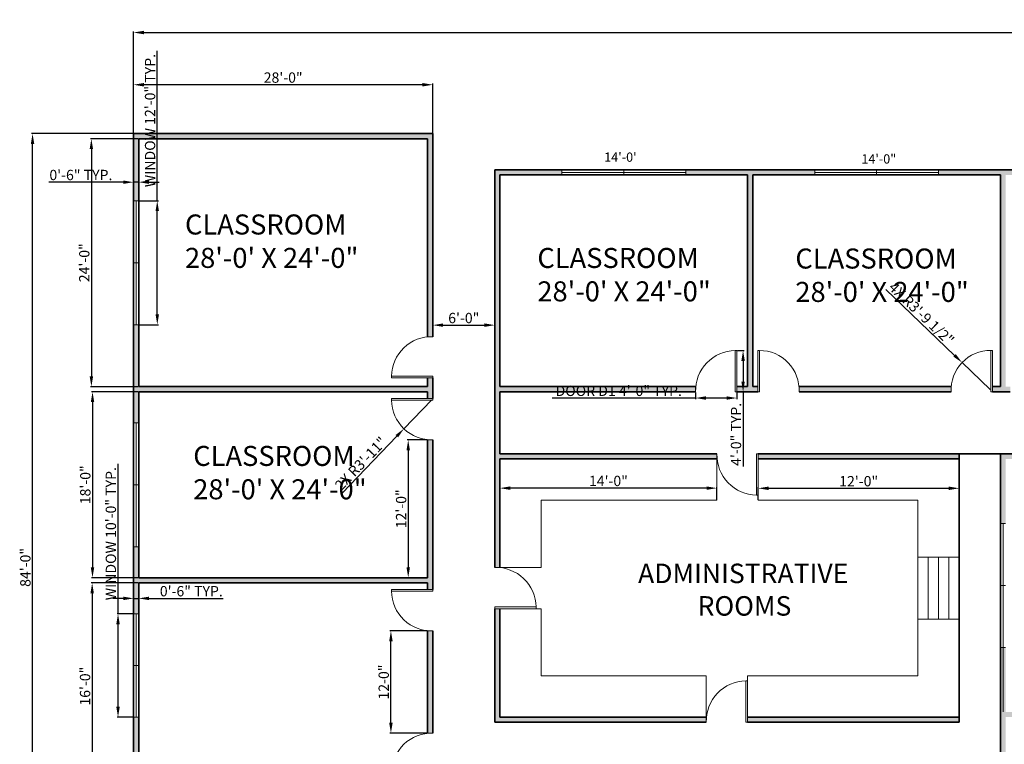
# Model space of a CAD drawing. Units: inches. Extents: x 2623 to 5095, y 1050 to 2384.
# Tile 2 of 4: x 2623 to 3768, y 1542 to 2384. Entities that reach past the tile are written whole.
import ezdxf

# ---------------------------------------------------------------- set-up
doc = ezdxf.new("R2010")
doc.units = ezdxf.units.IN
for name, color, linetype, lineweight in [('A-ANNO-DIMS', 2, 'Continuous', 13), ('A-ANNO-TEXT', 7, 'Continuous', 18), ('A-AREA-IDEN', 7, 'Continuous', 18), ('A-DOOR', 3, 'Continuous', 18), ('A-FLOR', 7, 'Continuous', 18), ('A-FLOR-STRS', 7, 'Continuous', 18), ('A-GLAZ', 4, 'Continuous', 18), ('A-WALL', 7, 'Continuous', 35)]:
    doc.layers.add(name, color=color, linetype=linetype, lineweight=lineweight)
doc.layers.add('A-WALL-PATT', color=251, linetype='Continuous', lineweight=9, true_color=0x636466)
doc.styles.get("Standard").update_dxf_attribs({"font": 'arial.ttf'})
doc.dimstyles.new('ISO-25', dxfattribs={"dimtxt": 12, "dimasz": 12, "dimexe": 1.25, "dimexo": 0.625, "dimtad": 1, "dimlunit": 3, "dimtxsty": 'Standard', "dimcen": 2.5, "dimadec": 0, "dimazin": 0, "dimtfac": 1, "dimtmove": 0, "dimatfit": 3, "dimfxl": 1, "dimarcsym": 0})

# ---------------------------------------------------------------- blocks, each defined once
blk = doc.blocks.new('*D8')
at = {"layer": 'A-ANNO-DIMS', "color": 0, "lineweight": -2, "transparency": 16777216}
for p, q in [((2755.7, 2252.2), (2755.7, 2309.7)), ((3091.7, 2308.4), (2767.7, 2308.4)), ((3103.7, 2252.2), (3103.7, 2309.7))]:
    blk.add_line(p, q, dxfattribs=at)
at = {"layer": 'A-ANNO-DIMS', "color": 0, "transparency": 16777216}
for points in [[(2767.7, 2310.4), (2767.7, 2306.4), (2755.7, 2308.4)], [(3091.7, 2310.4), (3091.7, 2306.4), (3103.7, 2308.4)]]:
    blk.add_solid(points, dxfattribs=at)
at = {"layer": 'Defpoints', "color": 0, "transparency": 16777216}
for p in [(2755.7, 2308.4), (2755.7, 2251.6), (3103.7, 2251.6)]:
    blk.add_point(p, dxfattribs=at)
at = {"layer": 'A-ANNO-DIMS', "color": 0, "transparency": 16777216, "insert": (2929.7, 2315.2), "char_height": 12, "attachment_point": 5}
blk.add_mtext('28\'-0"', dxfattribs=at)
blk = doc.blocks.new('*D9')
at = {"layer": 'A-ANNO-DIMS', "color": 0, "lineweight": -2, "transparency": 16777216}
for p, q in [((2761.1, 2245.6), (2705.5, 2245.6)), ((2706.7, 2233.6), (2706.7, 1969.6)), ((2761.1, 1957.6), (2705.5, 1957.6))]:
    blk.add_line(p, q, dxfattribs=at)
at = {"layer": 'A-ANNO-DIMS', "color": 0, "transparency": 16777216}
for points in [[(2704.7, 2233.6), (2708.7, 2233.6), (2706.7, 2245.6)], [(2704.7, 1969.6), (2708.7, 1969.6), (2706.7, 1957.6)]]:
    blk.add_solid(points, dxfattribs=at)
at = {"layer": 'Defpoints', "color": 0, "transparency": 16777216}
for p in [(2761.7, 2245.6), (2706.7, 1957.6), (2761.7, 1957.6)]:
    blk.add_point(p, dxfattribs=at)
at = {"layer": 'A-ANNO-DIMS', "color": 0, "transparency": 16777216, "insert": (2700, 2101.6), "char_height": 12, "attachment_point": 5, "rotation": 90}
blk.add_mtext('24\'-0"', dxfattribs=at)
blk = doc.blocks.new('*D10')
at = {"layer": 'A-ANNO-DIMS', "color": 0, "lineweight": -2, "transparency": 16777216}
for p, q in [((2761.1, 1951.6), (2706.7, 1951.6)), ((2708, 1939.6), (2708, 1747.6)), ((2761.1, 1735.6), (2706.7, 1735.6))]:
    blk.add_line(p, q, dxfattribs=at)
at = {"layer": 'A-ANNO-DIMS', "color": 0, "transparency": 16777216}
for points in [[(2706, 1939.6), (2710, 1939.6), (2708, 1951.6)], [(2706, 1747.6), (2710, 1747.6), (2708, 1735.6)]]:
    blk.add_solid(points, dxfattribs=at)
at = {"layer": 'Defpoints', "color": 0, "transparency": 16777216}
for p in [(2761.7, 1951.6), (2708, 1735.6), (2761.7, 1735.6)]:
    blk.add_point(p, dxfattribs=at)
at = {"layer": 'A-ANNO-DIMS', "color": 0, "transparency": 16777216, "insert": (2701.2, 1843.6), "char_height": 12, "attachment_point": 5, "rotation": 90}
blk.add_mtext('18\'-0"', dxfattribs=at)
blk = doc.blocks.new('*D11')
at = {"layer": 'A-ANNO-DIMS', "color": 0, "lineweight": -2, "transparency": 16777216}
for p, q in [((2761.1, 1729.6), (2706.4, 1729.6)), ((2707.6, 1717.6), (2707.6, 1501.6)), ((2761.1, 1489.6), (2706.4, 1489.6))]:
    blk.add_line(p, q, dxfattribs=at)
at = {"layer": 'A-ANNO-DIMS', "color": 0, "transparency": 16777216}
for points in [[(2705.6, 1717.6), (2709.6, 1717.6), (2707.6, 1729.6)], [(2705.6, 1501.6), (2709.6, 1501.6), (2707.6, 1489.6)]]:
    blk.add_solid(points, dxfattribs=at)
at = {"layer": 'Defpoints', "color": 0, "transparency": 16777216}
for p in [(2761.7, 1729.6), (2707.6, 1489.6), (2761.7, 1489.6)]:
    blk.add_point(p, dxfattribs=at)
at = {"layer": 'A-ANNO-DIMS', "color": 0, "transparency": 16777216, "insert": (2700.9, 1609.6), "char_height": 12, "attachment_point": 5, "rotation": 90}
blk.add_mtext('16\'-0"', dxfattribs=at)
blk = doc.blocks.new('*D22')
at = {"layer": 'A-ANNO-DIMS', "color": 0, "lineweight": -2, "transparency": 16777216}
for p, q in [((3097.1, 1895.7), (3073.9, 1895.7)), ((3075.1, 1883.7), (3075.1, 1747.6)), ((3097.1, 1735.6), (3073.9, 1735.6))]:
    blk.add_line(p, q, dxfattribs=at)
at = {"layer": 'A-ANNO-DIMS', "color": 0, "transparency": 16777216}
for points in [[(3073.1, 1883.7), (3077.1, 1883.7), (3075.1, 1895.7)], [(3073.1, 1747.6), (3077.1, 1747.6), (3075.1, 1735.6)]]:
    blk.add_solid(points, dxfattribs=at)
at = {"layer": 'Defpoints', "color": 0, "transparency": 16777216}
for p in [(3097.7, 1895.7), (3075.1, 1735.6), (3097.7, 1735.6)]:
    blk.add_point(p, dxfattribs=at)
at = {"layer": 'A-ANNO-DIMS', "color": 0, "transparency": 16777216, "insert": (3068.4, 1815.7), "char_height": 12, "attachment_point": 5, "rotation": 90}
blk.add_mtext('12\'-0"', dxfattribs=at)
blk = doc.blocks.new('*D23')
at = {"layer": 'A-ANNO-DIMS', "color": 0, "lineweight": -2, "transparency": 16777216}
for p, q in [((3103.7, 2016.3), (3103.7, 2030.3)), ((3115.7, 2029.1), (3163.7, 2029.1)), ((3175.7, 2016.3), (3175.7, 2030.3))]:
    blk.add_line(p, q, dxfattribs=at)
at = {"layer": 'A-ANNO-DIMS', "color": 0, "transparency": 16777216}
for points in [[(3115.7, 2031.1), (3115.7, 2027.1), (3103.7, 2029.1)], [(3163.7, 2031.1), (3163.7, 2027.1), (3175.7, 2029.1)]]:
    blk.add_solid(points, dxfattribs=at)
at = {"layer": 'Defpoints', "color": 0, "transparency": 16777216}
for p in [(3175.7, 2029.1), (3103.7, 2015.7), (3175.7, 2015.7)]:
    blk.add_point(p, dxfattribs=at)
at = {"layer": 'A-ANNO-DIMS', "color": 0, "transparency": 16777216, "insert": (3139.7, 2035.8), "char_height": 12, "attachment_point": 5}
blk.add_mtext('6\'-0"', dxfattribs=at)
blk = doc.blocks.new('*D24')
at = {"layer": 'A-ANNO-DIMS', "color": 0, "lineweight": -2, "transparency": 16777216}
for p, q in [((3097.1, 1673.8), (3053.7, 1673.8)), ((3055, 1567), (3055, 1661.8)), ((3097.1, 1555), (3053.7, 1555))]:
    blk.add_line(p, q, dxfattribs=at)
at = {"layer": 'A-ANNO-DIMS', "color": 0, "transparency": 16777216}
for points in [[(3053, 1661.8), (3057, 1661.8), (3055, 1673.8)], [(3053, 1567), (3057, 1567), (3055, 1555)]]:
    blk.add_solid(points, dxfattribs=at)
at = {"layer": 'Defpoints', "color": 0, "transparency": 16777216}
for p in [(3055, 1673.8), (3097.7, 1673.8), (3097.7, 1555)]:
    blk.add_point(p, dxfattribs=at)
at = {"layer": 'A-ANNO-DIMS', "color": 0, "transparency": 16777216, "insert": (3048.2, 1614.4), "char_height": 12, "attachment_point": 5, "rotation": 90}
blk.add_mtext('12-0"', dxfattribs=at)
blk = doc.blocks.new('*D39')
at = {"layer": 'A-ANNO-DIMS', "color": 0, "lineweight": -2, "transparency": 16777216}
for p, q in [((3482.1, 1826.2), (3482.1, 1840.7)), ((3494.1, 1839.5), (3703.7, 1839.5)), ((3715.7, 1826.2), (3715.7, 1840.7))]:
    blk.add_line(p, q, dxfattribs=at)
at = {"layer": 'A-ANNO-DIMS', "color": 0, "transparency": 16777216}
for points in [[(3494.1, 1841.5), (3494.1, 1837.5), (3482.1, 1839.5)], [(3703.7, 1841.5), (3703.7, 1837.5), (3715.7, 1839.5)]]:
    blk.add_solid(points, dxfattribs=at)
at = {"layer": 'Defpoints', "color": 0, "transparency": 16777216}
for p in [(3715.7, 1839.5), (3482.1, 1825.6), (3715.7, 1825.6)]:
    blk.add_point(p, dxfattribs=at)
at = {"layer": 'A-ANNO-DIMS', "color": 0, "transparency": 16777216, "insert": (3598.9, 1846.2), "char_height": 12, "attachment_point": 5}
blk.add_mtext('12\'-0"', dxfattribs=at)
blk = doc.blocks.new('*D40')
at = {"layer": 'A-ANNO-DIMS', "color": 0, "lineweight": -2, "transparency": 16777216}
for p, q in [((3181.7, 1826.2), (3181.7, 1841)), ((3422.1, 1839.7), (3193.7, 1839.7)), ((3434.1, 1826.2), (3434.1, 1841))]:
    blk.add_line(p, q, dxfattribs=at)
at = {"layer": 'A-ANNO-DIMS', "color": 0, "transparency": 16777216}
for points in [[(3193.7, 1841.7), (3193.7, 1837.7), (3181.7, 1839.7)], [(3422.1, 1841.7), (3422.1, 1837.7), (3434.1, 1839.7)]]:
    blk.add_solid(points, dxfattribs=at)
at = {"layer": 'Defpoints', "color": 0, "transparency": 16777216}
for p in [(3181.7, 1839.7), (3181.7, 1825.6), (3434.1, 1825.6)]:
    blk.add_point(p, dxfattribs=at)
at = {"layer": 'A-ANNO-DIMS', "color": 0, "transparency": 16777216, "insert": (3307.9, 1846.5), "char_height": 12, "attachment_point": 5}
blk.add_mtext('14\'-0"', dxfattribs=at)
blk = doc.blocks.new('WIN-144-DOUBLE-LIGHT')
for p, q in [((0, 6), (0, 0)), ((144, 3), (0, 3)), ((72, 6), (72, 0)), ((144, 6), (144, 0))]:
    blk.add_line(p, q)
blk = doc.blocks.new('WIN-120-DOUBLE-LIGHT')
for p, q in [((6, 120), (0, 120)), ((3, 120), (3, 0)), ((6, 60), (0, 60)), ((6, 0), (0, 0))]:
    blk.add_line(p, q)
blk = doc.blocks.new('DOOR-48-LEAF-AND-JAMBS')
for p, q in [((0, 48), (0, 0)), ((2, 48), (0, 48)), ((0, 48), (0, 42)), ((2, 0), (2, 48)), ((48, 48), (48, 42)), ((0, 0), (2, 0))]:
    blk.add_line(p, q)
blk = doc.blocks.new('*D49')
at = {"layer": 'A-ANNO-DIMS', "color": 0, "lineweight": -2, "transparency": 16777216}
for p, q in [((3409.3, 1951), (3409.3, 1943.2)), ((3457.3, 1951), (3457.3, 1943.2)), ((3409.3, 1944.4), (3242.5, 1944.4)), ((3445.3, 1944.4), (3421.3, 1944.4))]:
    blk.add_line(p, q, dxfattribs=at)
at = {"layer": 'A-ANNO-DIMS', "color": 0, "transparency": 16777216}
for points in [[(3421.3, 1946.4), (3421.3, 1942.4), (3409.3, 1944.4)], [(3445.3, 1946.4), (3445.3, 1942.4), (3457.3, 1944.4)]]:
    blk.add_solid(points, dxfattribs=at)
at = {"layer": 'Defpoints', "color": 0, "transparency": 16777216}
for p in [(3409.3, 1951.6), (3457.3, 1951.6), (3409.3, 1944.4)]:
    blk.add_point(p, dxfattribs=at)
at = {"layer": 'A-ANNO-DIMS', "color": 0, "transparency": 16777216, "insert": (3319.9, 1951.2), "char_height": 12, "attachment_point": 5}
blk.add_mtext('DOOR D1 4\'-0" TYP.', dxfattribs=at)
blk = doc.blocks.new('*D50')
at = {"layer": 'A-ANNO-DIMS', "color": 0, "lineweight": -2, "transparency": 16777216}
for p, q in [((3457.9, 1999.6), (3465.8, 1999.6)), ((3464.5, 1987.6), (3464.5, 1963.6)), ((3457.9, 1951.6), (3465.8, 1951.6)), ((3464.5, 1951.6), (3464.5, 1864.7))]:
    blk.add_line(p, q, dxfattribs=at)
at = {"layer": 'A-ANNO-DIMS', "color": 0, "transparency": 16777216}
for points in [[(3462.5, 1987.6), (3466.5, 1987.6), (3464.5, 1999.6)], [(3462.5, 1963.6), (3466.5, 1963.6), (3464.5, 1951.6)]]:
    blk.add_solid(points, dxfattribs=at)
at = {"layer": 'Defpoints', "color": 0, "transparency": 16777216}
for p in [(3457.3, 1999.6), (3457.3, 1951.6), (3464.5, 1951.6)]:
    blk.add_point(p, dxfattribs=at)
at = {"layer": 'A-ANNO-DIMS', "color": 0, "transparency": 16777216, "insert": (3457.8, 1902.2), "char_height": 12, "attachment_point": 5, "rotation": 90}
blk.add_mtext('4\'-0" TYP.', dxfattribs=at)
blk = doc.blocks.new('*D51')
at = {"layer": 'A-ANNO-DIMS', "color": 0, "lineweight": -2, "transparency": 16777216}
for p, q in [((2783.3, 2173.6), (2783.3, 2348)), ((2762.3, 2173.6), (2784.6, 2173.6)), ((2783.3, 2041.6), (2783.3, 2161.6)), ((2762.3, 2029.6), (2784.6, 2029.6))]:
    blk.add_line(p, q, dxfattribs=at)
at = {"layer": 'A-ANNO-DIMS', "color": 0, "transparency": 16777216}
for points in [[(2781.3, 2161.6), (2785.3, 2161.6), (2783.3, 2173.6)], [(2781.3, 2041.6), (2785.3, 2041.6), (2783.3, 2029.6)]]:
    blk.add_solid(points, dxfattribs=at)
at = {"layer": 'Defpoints', "color": 0, "transparency": 16777216}
for p in [(2761.7, 2173.6), (2783.3, 2173.6), (2761.7, 2029.6)]:
    blk.add_point(p, dxfattribs=at)
at = {"layer": 'A-ANNO-DIMS', "color": 0, "transparency": 16777216, "insert": (2776.5, 2266.8), "char_height": 12, "attachment_point": 5, "rotation": 90}
blk.add_mtext('WINDOW 12\'-0" TYP.', dxfattribs=at)
blk = doc.blocks.new('*D52')
at = {"layer": 'A-ANNO-DIMS', "color": 0, "lineweight": -2, "transparency": 16777216}
for p, q in [((2743.7, 2195.2), (2657.3, 2195.2)), ((2755.7, 2174.2), (2755.7, 2196.5)), ((2761.7, 2195.2), (2755.7, 2195.2)), ((2761.7, 2174.2), (2761.7, 2196.5)), ((2773.7, 2195.2), (2785.7, 2195.2))]:
    blk.add_line(p, q, dxfattribs=at)
at = {"layer": 'A-ANNO-DIMS', "color": 0, "transparency": 16777216}
for points in [[(2743.7, 2197.2), (2743.7, 2193.2), (2755.7, 2195.2)], [(2773.7, 2197.2), (2773.7, 2193.2), (2761.7, 2195.2)]]:
    blk.add_solid(points, dxfattribs=at)
at = {"layer": 'Defpoints', "color": 0, "transparency": 16777216}
for p in [(2755.7, 2195.2), (2755.7, 2173.6), (2761.7, 2173.6)]:
    blk.add_point(p, dxfattribs=at)
at = {"layer": 'A-ANNO-DIMS', "color": 0, "transparency": 16777216, "insert": (2694.5, 2202), "char_height": 12, "attachment_point": 5}
blk.add_mtext('0\'-6" TYP.', dxfattribs=at)
blk = doc.blocks.new('*D55')
at = {"layer": 'A-ANNO-DIMS', "color": 0, "lineweight": -2, "transparency": 16777216}
for p, q in [((2737.7, 1693.6), (2737.7, 1868)), ((2755.1, 1693.6), (2736.5, 1693.6)), ((2737.7, 1585.6), (2737.7, 1681.6)), ((2755.1, 1573.6), (2736.5, 1573.6))]:
    blk.add_line(p, q, dxfattribs=at)
at = {"layer": 'A-ANNO-DIMS', "color": 0, "transparency": 16777216}
for points in [[(2735.7, 1681.6), (2739.7, 1681.6), (2737.7, 1693.6)], [(2735.7, 1585.6), (2739.7, 1585.6), (2737.7, 1573.6)]]:
    blk.add_solid(points, dxfattribs=at)
at = {"layer": 'Defpoints', "color": 0, "transparency": 16777216}
for p in [(2737.7, 1693.6), (2755.7, 1693.6), (2755.7, 1573.6)]:
    blk.add_point(p, dxfattribs=at)
at = {"layer": 'A-ANNO-DIMS', "color": 0, "transparency": 16777216, "insert": (2730.9, 1786.8), "char_height": 12, "attachment_point": 5, "rotation": 90}
blk.add_mtext('WINDOW 10\'-0" TYP.', dxfattribs=at)
blk = doc.blocks.new('*D56')
at = {"layer": 'A-ANNO-DIMS', "color": 0, "lineweight": -2, "transparency": 16777216}
for p, q in [((2743.7, 1711.6), (2731.7, 1711.6)), ((2755.7, 1694.2), (2755.7, 1712.9)), ((2755.7, 1711.6), (2761.7, 1711.6)), ((2761.7, 1694.2), (2761.7, 1712.9)), ((2773.7, 1711.6), (2860.1, 1711.6))]:
    blk.add_line(p, q, dxfattribs=at)
at = {"layer": 'A-ANNO-DIMS', "color": 0, "transparency": 16777216}
for points in [[(2743.7, 1713.6), (2743.7, 1709.6), (2755.7, 1711.6)], [(2773.7, 1713.6), (2773.7, 1709.6), (2761.7, 1711.6)]]:
    blk.add_solid(points, dxfattribs=at)
at = {"layer": 'Defpoints', "color": 0, "transparency": 16777216}
for p in [(2761.7, 1711.6), (2755.7, 1693.6), (2761.7, 1693.6)]:
    blk.add_point(p, dxfattribs=at)
at = {"layer": 'A-ANNO-DIMS', "color": 0, "transparency": 16777216, "insert": (2822.9, 1718.4), "char_height": 12, "attachment_point": 5}
blk.add_mtext('0\'-6" TYP.', dxfattribs=at)
blk = doc.blocks.new('*D65')
at = {"layer": 'A-ANNO-DIMS', "color": 0, "lineweight": -2, "transparency": 16777216}
for p, q in [((2755.7, 2252.2), (2755.7, 2370.3)), ((4975.7, 2138.2), (4975.7, 2370.3)), ((2767.7, 2369.1), (4963.7, 2369.1))]:
    blk.add_line(p, q, dxfattribs=at)
at = {"layer": 'A-ANNO-DIMS', "color": 0, "transparency": 16777216}
for points in [[(2767.7, 2371.1), (2767.7, 2367.1), (2755.7, 2369.1)], [(4963.7, 2371.1), (4963.7, 2367.1), (4975.7, 2369.1)]]:
    blk.add_solid(points, dxfattribs=at)
at = {"layer": 'Defpoints', "color": 0, "transparency": 16777216}
for p in [(4975.7, 2369.1), (2755.7, 2251.6), (4975.7, 2137.6)]:
    blk.add_point(p, dxfattribs=at)
at = {"layer": 'A-ANNO-DIMS', "color": 0, "transparency": 16777216, "insert": (3865.7, 2375.8), "char_height": 12, "attachment_point": 5}
blk.add_mtext('185\'-0"', dxfattribs=at)
blk = doc.blocks.new('*D66')
at = {"layer": 'A-ANNO-DIMS', "color": 0, "lineweight": -2, "transparency": 16777216}
for p, q in [((2755.1, 2251.6), (2637, 2251.6)), ((2638.3, 1255.6), (2638.3, 2239.6)), ((2755.1, 1243.6), (2637, 1243.6))]:
    blk.add_line(p, q, dxfattribs=at)
at = {"layer": 'A-ANNO-DIMS', "color": 0, "transparency": 16777216}
for points in [[(2636.3, 2239.6), (2640.3, 2239.6), (2638.3, 2251.6)], [(2636.3, 1255.6), (2640.3, 1255.6), (2638.3, 1243.6)]]:
    blk.add_solid(points, dxfattribs=at)
at = {"layer": 'Defpoints', "color": 0, "transparency": 16777216}
for p in [(2638.3, 2251.6), (2755.7, 2251.6), (2755.7, 1243.6)]:
    blk.add_point(p, dxfattribs=at)
at = {"layer": 'A-ANNO-DIMS', "color": 0, "transparency": 16777216, "insert": (2631.5, 1747.6), "char_height": 12, "attachment_point": 5, "rotation": 90}
blk.add_mtext('84\'-0"', dxfattribs=at)
blk = doc.blocks.new('*D70')
at = {"layer": 'A-ANNO-DIMS', "color": 0, "lineweight": -2, "transparency": 16777216}
for p, q in [((3102.5, 1942.5), (3070.1, 1908.7)), ((2998.2, 1833.7), (3061.8, 1900.1))]:
    blk.add_line(p, q, dxfattribs=at)
at = {"layer": 'A-ANNO-DIMS', "color": 0, "transparency": 16777216}
blk.add_solid([(3060.4, 1901.5), (3063.3, 1898.7), (3070.1, 1908.7)], dxfattribs=at)
at = {"layer": 'Defpoints', "color": 0, "transparency": 16777216}
for p in [(3102.5, 1942.5), (3070.1, 1908.7)]:
    blk.add_point(p, dxfattribs=at)
at = {"layer": 'A-ANNO-DIMS', "color": 0, "transparency": 16777216, "insert": (3021, 1867.2), "char_height": 12, "attachment_point": 5, "rotation": 46.2193}
blk.add_mtext('2X R3\'-11"', dxfattribs=at)
blk = doc.blocks.new('*D73')
at = {"layer": 'A-ANNO-DIMS', "color": 0, "lineweight": -2, "transparency": 16777216}
for p, q in [((3630.4, 2070.7), (3710.4, 1994)), ((3751.8, 1954.4), (3719.1, 1985.7))]:
    blk.add_line(p, q, dxfattribs=at)
at = {"layer": 'A-ANNO-DIMS', "color": 0, "transparency": 16777216}
blk.add_solid([(3711.8, 1995.4), (3709, 1992.5), (3719.1, 1985.7)], dxfattribs=at)
at = {"layer": 'Defpoints', "color": 0, "transparency": 16777216}
for p in [(3719.1, 1985.7), (3751.8, 1954.4)]:
    blk.add_point(p, dxfattribs=at)
at = {"layer": 'A-ANNO-DIMS', "color": 0, "transparency": 16777216, "insert": (3670.8, 2041.4), "char_height": 12, "attachment_point": 5, "rotation": 316.2187}
blk.add_mtext('4X R3\'-9 1/2"', dxfattribs=at)

msp = doc.modelspace()

# ---------------------------------------------------------------- hatches: boundary and pattern name
at = {"layer": 'A-WALL-PATT'}
h = msp.add_hatch(color=256, dxfattribs=at)
h.dxf.hatch_style = 1
h.paths.add_polyline_path([(3103.717, 2251.615), (2755.717, 2251.615), (2755.717, 2173.615), (2761.717, 2173.615), (2761.717, 2245.615), (3097.717, 2245.615), (3097.717, 2015.688), (3100.811, 2015.688, -0.01561511), (3103.717, 2015.688)])
h.paths.add_polyline_path([(3103.717, 1967.688), (3097.717, 1967.688), (3097.717, 1957.615), (2761.717, 1957.615), (2761.717, 2029.615), (2755.717, 2029.615), (2755.717, 1915.615), (2761.717, 1915.615), (2761.717, 1951.615), (3097.717, 1951.615), (3097.717, 1943.747), (3103.717, 1943.747)])
h.paths.add_polyline_path([(3103.717, 1895.747, -0.01327118), (3101.235, 1895.747), (3097.717, 1895.747), (3097.717, 1735.615), (2761.717, 1735.615), (2761.717, 1771.615), (2755.717, 1771.615), (2755.717, 1693.615), (2761.717, 1693.615), (2761.717, 1729.615), (3097.717, 1729.615), (3097.717, 1721.81), (3103.717, 1721.81)])
h.paths.add_polyline_path([(2761.717, 1573.615), (2755.717, 1573.615), (2755.717, 1405.615), (2761.717, 1405.615)])
h.paths.add_polyline_path([(2761.717, 1285.615), (2755.717, 1285.615), (2755.717, 1243.615), (2857.717, 1243.615), (2857.717, 1249.615), (2761.717, 1249.615)])
h.paths.add_polyline_path([(3152.017, 1249.615), (3103.717, 1249.615), (3103.717, 1489.615), (3237.319, 1489.615, -0.03349431), (3237.344, 1495.615), (3103.717, 1495.615), (3103.717, 1507.046), (3097.717, 1507.046), (3097.717, 1249.615), (3001.717, 1249.615), (3001.717, 1243.615), (3103.717, 1243.615), (3152.017, 1243.615)])
h.paths.add_polyline_path([(3103.717, 1673.81, -0.01537929), (3100.853, 1673.81), (3097.717, 1673.81), (3097.717, 1555.046), (3101.163, 1555.046, -0.01366836), (3103.717, 1555.046)])
h.paths.add_polyline_path([(3302.317, 1249.615), (3302.317, 1297.615), (3385.117, 1297.615), (3385.117, 1303.615), (3302.317, 1303.615), (3302.317, 1489.615), (3503.954, 1489.615), (3503.954, 1492.911, -0.01449155), (3503.954, 1495.615), (3285.344, 1495.615), (3285.344, 1489.615), (3296.317, 1489.615), (3296.317, 1249.615), (3248.017, 1249.615), (3248.017, 1243.615), (3302.317, 1243.615)])
h.paths.add_polyline_path([(3569.917, 1489.615), (3579.094, 1489.615), (3579.094, 1495.615), (3551.954, 1495.615), (3551.954, 1489.615), (3563.917, 1489.615), (3563.917, 1303.615), (3481.117, 1303.615), (3481.117, 1297.615), (3563.917, 1297.615), (3563.917, 1249.615), (3563.917, 1243.615), (3618.817, 1243.615), (3618.817, 1249.615), (3569.917, 1249.615)])
h.paths.add_polyline_path([(3846.517, 1249.615), (3769.717, 1249.615), (3769.717, 1573.615), (3846.517, 1573.615), (3846.517, 1579.615), (3769.717, 1579.615), (3769.717, 1654.615), (3763.717, 1654.615), (3763.717, 1495.615), (3627.094, 1495.615, -0.01677945), (3627.094, 1492.499), (3627.094, 1489.615), (3763.717, 1489.615), (3763.717, 1249.615), (3714.817, 1249.615), (3714.817, 1243.615), (3763.717, 1243.615), (3846.517, 1243.615)])
h.paths.add_polyline_path([(4084.941, 1249.615), (4073.317, 1249.615), (4073.317, 1305.13), (4067.317, 1305.13), (4067.317, 1249.615), (3990.517, 1249.615), (3990.517, 1243.615), (4084.941, 1243.615)])
h.paths.add_polyline_path([(4277.411, 1249.615), (4208.317, 1249.615), (4208.317, 1366.615), (4282.724, 1366.615), (4282.724, 1370.675, -0.01031167), (4282.724, 1372.615), (4115.317, 1372.615), (4115.317, 1381.792), (4114.62, 1381.792, -0.02925374), (4109.317, 1381.792), (4109.317, 1372.615), (4073.317, 1372.615), (4067.317, 1372.615), (4067.317, 1353.13), (4073.317, 1353.13), (4073.317, 1366.615), (4202.317, 1366.615), (4202.317, 1249.615), (4120.941, 1249.615), (4120.941, 1243.615), (4277.411, 1243.615)])
h.paths.add_polyline_path([(4939.717, 1300.615), (4933.717, 1300.615), (4818.498, 1300.615), (4818.498, 1294.615), (4933.717, 1294.615), (4933.717, 1249.615), (4349.317, 1249.615), (4349.317, 1294.615), (4465.249, 1294.615), (4465.249, 1300.615), (4349.317, 1300.615), (4349.317, 1573.615), (4430.317, 1573.615), (4430.317, 1579.615), (4358.917, 1579.615), (4358.917, 1873.615), (4365.566, 1873.615), (4365.566, 1879.615), (4345.539, 1879.615), (4345.539, 1873.615), (4352.917, 1873.615), (4352.917, 1579.615), (4282.117, 1579.615), (4282.117, 1573.615), (4343.317, 1573.615), (4343.317, 1456.615), (4177.166, 1456.615), (4177.166, 1450.615), (4343.317, 1450.615), (4343.317, 1372.615), (4330.724, 1372.615), (4330.724, 1366.615), (4343.317, 1366.615), (4343.317, 1249.615), (4313.411, 1249.615), (4313.411, 1243.615), (4939.717, 1243.615)])
h = msp.add_hatch(color=256, dxfattribs=at)
h.dxf.hatch_style = 1
h.paths.add_polyline_path([(4651.717, 1615.615), (4975.717, 1615.615), (4975.717, 1657.615), (4969.717, 1657.615), (4969.717, 1621.615), (4729.717, 1621.615), (4729.717, 1741.615), (4735.396, 1741.615), (4735.396, 1747.615), (4723.717, 1747.615), (4723.717, 1621.615), (4651.717, 1621.615), (4651.717, 1654.615), (4645.717, 1654.615), (4645.717, 1579.615), (4574.317, 1579.615), (4574.317, 1573.615), (4651.717, 1573.615)])
h.paths.add_polyline_path([(4939.717, 1579.615), (4864.717, 1579.615), (4864.717, 1573.615), (4933.717, 1573.615), (4933.717, 1345.615), (4939.717, 1345.615)])
h.paths.add_polyline_path([(4975.717, 1804.615), (4969.717, 1804.615), (4969.717, 1747.615), (4783.396, 1747.615, -0.01744529), (4783.396, 1744.379), (4783.396, 1741.615), (4969.717, 1741.615), (4969.717, 1705.615), (4975.717, 1705.615)])
h.paths.add_polyline_path([(4975.717, 2047.615), (4969.717, 2047.615), (4969.717, 2011.615), (4785.608, 2011.615), (4785.608, 2008.9, -0.01771988), (4785.608, 2005.615), (4969.717, 2005.615), (4969.717, 1948.615), (4975.717, 1948.615), (4975.717, 2005.615)])
h.paths.add_polyline_path([(4975.717, 2137.615), (4729.717, 2137.615), (4723.717, 2137.615), (4723.717, 2005.615), (4737.608, 2005.615), (4737.608, 2011.615), (4729.717, 2011.615), (4729.717, 2131.615), (4969.717, 2131.615), (4969.717, 2095.615), (4975.717, 2095.615)])
h.paths.add_polyline_path([(4651.717, 2209.615), (4573.717, 2209.615), (4573.717, 2203.615), (4645.717, 2203.615), (4645.717, 2128.615), (4651.717, 2128.615)])
h.paths.add_polyline_path([(4651.717, 2032.615), (4645.717, 2032.615), (4645.717, 1957.615), (4413.911, 1957.615), (4413.911, 1956.398, -0.02623296), (4413.911, 1951.615), (4651.717, 1951.615)])
h.paths.add_polyline_path([(4357.717, 2203.615), (4429.717, 2203.615), (4429.717, 2209.615), (4279.717, 2209.615), (4279.717, 2203.615), (4351.717, 2203.615), (4351.717, 1957.615), (4345.154, 1957.615), (4345.154, 1951.615), (4365.911, 1951.615), (4365.911, 1957.615), (4357.717, 1957.615)])
h.paths.add_polyline_path([(4063.717, 2203.615), (4135.717, 2203.615), (4135.717, 2209.615), (3985.717, 2209.615), (3985.717, 2203.615), (4057.717, 2203.615), (4057.717, 1957.615), (3823.079, 1957.615), (3823.079, 1955.024, -0.01841239), (3823.079, 1951.615), (4075.656, 1951.615), (4075.656, 1957.615), (4063.717, 1957.615)])
h.paths.add_polyline_path([(4297.09, 1957.615), (4123.656, 1957.615), (4123.656, 1954.68, -0.01649439), (4123.656, 1951.615), (4297.154, 1951.615, -0.03370804)])
h.paths.add_polyline_path([(3769.717, 2203.615), (3841.717, 2203.615), (3841.717, 2209.615), (3691.717, 2209.615), (3691.717, 2203.615), (3763.717, 2203.615), (3763.717, 1957.615), (3754.594, 1957.615), (3754.594, 1951.615), (3775.079, 1951.615), (3775.079, 1957.615), (3769.717, 1957.615)])
h.paths.add_polyline_path([(3706.594, 1957.102), (3706.594, 1957.615), (3529.616, 1957.615), (3529.616, 1955.888, -0.02330465), (3529.616, 1951.615), (3706.594, 1951.615, -0.03033114)])
h.paths.add_polyline_path([(3481.616, 1957.615), (3475.717, 1957.615), (3475.717, 2203.615), (3547.717, 2203.615), (3547.717, 2209.615), (3397.717, 2209.615), (3397.717, 2203.615), (3469.717, 2203.615), (3469.717, 1957.615), (3457.307, 1957.615), (3457.307, 1951.615), (3481.616, 1951.615)])
h.paths.add_polyline_path([(3409.307, 1954.491), (3409.307, 1957.615), (3181.717, 1957.615), (3181.717, 2203.615), (3253.717, 2203.615), (3253.717, 2209.615), (3175.717, 2209.615), (3175.717, 1747.615, -0.01406848), (3178.344, 1747.615), (3181.717, 1747.615), (3181.717, 1873.615), (3434.065, 1873.615), (3434.065, 1877.049, -0.01373428), (3434.065, 1879.615), (3181.717, 1879.615), (3181.717, 1951.615), (3409.307, 1951.615, -0.01544691)])
h.paths.add_polyline_path([(4651.717, 1879.615), (4413.566, 1879.615, -0.01934194), (4413.566, 1876.041), (4413.566, 1873.615), (4645.717, 1873.615), (4645.717, 1798.615), (4651.717, 1798.615)])
h.paths.add_polyline_path([(4138.117, 1579.615), (4067.317, 1579.615), (4067.317, 1873.615), (4073.262, 1873.615), (4073.262, 1879.615), (4055.249, 1879.615), (4055.249, 1873.615), (4061.317, 1873.615), (4061.317, 1579.615), (3990.517, 1579.615), (3990.517, 1573.615), (4067.317, 1573.615), (4067.317, 1450.615), (4109.317, 1450.615), (4109.317, 1429.792), (4115.317, 1429.792), (4115.317, 1450.615), (4129.166, 1450.615), (4129.166, 1456.615), (4073.317, 1456.615), (4073.317, 1573.615), (4138.117, 1573.615)])
h.paths.add_polyline_path([(4297.539, 1879.615), (4121.262, 1879.615, -0.02641892), (4121.262, 1874.8), (4121.262, 1873.615), (4297.539, 1873.615), (4297.539, 1876.326, -0.01774472)])
h.paths.add_polyline_path([(4007.249, 1879.615), (3763.717, 1879.615), (3763.717, 1798.615), (3769.717, 1798.615), (3769.717, 1873.615), (4007.249, 1873.615), (4007.249, 1876.064, -0.01921077)])
h.paths.add_polyline_path([(3715.717, 1573.615), (3469.717, 1573.615), (3469.717, 1567.615), (3715.717, 1567.615)])
h.paths.add_polyline_path([(3421.717, 1570.87), (3421.717, 1573.615), (3181.717, 1573.615), (3181.717, 1699.615), (3175.717, 1699.615), (3175.717, 1567.615), (3421.717, 1567.615, -0.01755055)])
h.paths.add_polyline_path([(3715.717, 1879.615), (3482.065, 1879.615), (3482.065, 1873.615), (3715.717, 1873.615)])

# ---------------------------------------------------------------- linework, layer by layer
at = {"layer": 'A-DOOR'}
for centre, radius, start, end in [((3102.264, 1969.161), 46.55, 88.210786, 179.351463), ((3455.85, 1953.053), 46.565, 90.667806, 181.769945), ((3483.802, 1953.751), 45.864, 357.329967, 90.232282), ((3751.775, 1954.358), 45.264, 88.963123, 183.474627), ((3102.476, 1942.496), 46.765, 180.917075, 271.520676), ((3480.77, 1878.332), 46.722, 178.426267, 269.135983), ((3177.031, 1700.942), 46.691, 0.825728, 91.612022), ((3102.285, 1720.359), 46.571, 180.675552, 271.762198), ((3468.063, 1569.242), 46.374, 90.426812, 182.010939), ((3102.44, 1508.335), 46.728, 88.433819, 179.12843)]:
    msp.add_arc(centre, radius, start, end, dxfattribs=at)
at = {"layer": 'A-FLOR'}
for p, q in [((3434.065, 1825.615), (3434.065, 1873.615)), ((3482.065, 1825.615), (3482.065, 1833.987)), ((3229.717, 1825.615), (3434.065, 1825.615)), ((3229.717, 1825.615), (3229.717, 1747.615)), ((3482.065, 1825.615), (3667.717, 1825.615)), ((3667.717, 1825.615), (3667.717, 1621.615)), ((3229.717, 1747.615), (3181.717, 1747.615)), ((3229.717, 1699.615), (3223.717, 1699.615)), ((3229.717, 1699.615), (3229.717, 1621.615)), ((3229.717, 1621.615), (3421.717, 1621.615)), ((3421.717, 1621.615), (3421.717, 1570.615)), ((3469.717, 1621.615), (3667.717, 1621.615)), ((3469.717, 1621.615), (3469.717, 1615.615))]:
    msp.add_line(p, q, dxfattribs=at)
at = {"layer": 'A-FLOR-STRS'}
for p, q in [((3667.717, 1759.615), (3715.717, 1759.615)), ((3679.717, 1759.615), (3679.717, 1687.615)), ((3691.717, 1759.615), (3691.717, 1687.615)), ((3703.717, 1759.615), (3703.717, 1687.615)), ((3667.717, 1687.615), (3715.717, 1687.615))]:
    msp.add_line(p, q, dxfattribs=at)
at = {"layer": 'A-GLAZ'}
for p, q in [((3769.717, 1798.615), (3763.717, 1798.615)), ((3766.717, 1798.615), (3766.717, 1579.615)), ((3769.717, 1726.615), (3763.717, 1726.615)), ((2761.717, 1693.615), (2755.717, 1693.615)), ((2761.717, 1693.615), (2755.717, 1693.615)), ((3769.717, 1654.615), (3763.717, 1654.615))]:
    msp.add_line(p, q, dxfattribs=at)
at = {"layer": 'A-WALL'}
for p, q in [((2755.717, 2251.615), (3103.717, 2251.615)), ((2755.717, 1243.615), (2755.717, 2251.615)), ((2761.717, 2245.615), (3097.717, 2245.615)), ((2761.717, 1957.615), (2761.717, 2245.615)), ((3097.717, 2245.615), (3097.717, 2015.688)), ((3103.717, 2251.615), (3103.717, 2015.688)), ((3175.717, 2209.615), (3175.717, 1747.615)), ((3175.717, 2209.615), (4651.717, 2209.615)), ((3181.717, 2203.615), (3181.717, 1957.615)), ((3181.717, 2203.615), (3469.717, 2203.615)), ((3469.717, 2203.615), (3469.717, 1957.615)), ((3475.717, 2203.615), (3475.717, 1957.615)), ((3475.717, 2203.615), (3763.717, 2203.615)), ((3763.717, 2203.615), (3763.717, 1957.615)), ((3097.717, 1967.688), (3097.717, 1957.615)), ((3103.717, 1967.688), (3103.717, 1943.747)), ((3097.717, 1957.615), (2761.717, 1957.615)), ((3097.717, 1951.615), (2761.717, 1951.615)), ((2761.717, 1951.615), (2761.717, 1735.615)), ((3097.717, 1951.615), (3097.717, 1943.747)), ((3409.307, 1957.615), (3181.717, 1957.615)), ((3181.717, 1951.615), (3409.307, 1951.615)), ((3181.717, 1951.615), (3181.717, 1879.615)), ((3469.717, 1957.615), (3457.307, 1957.615)), ((3457.307, 1951.615), (3481.616, 1951.615)), ((3475.717, 1957.615), (3481.616, 1957.615)), ((3529.616, 1957.615), (3706.594, 1957.615)), ((3529.616, 1951.615), (3706.594, 1951.615)), ((3754.594, 1957.615), (3763.717, 1957.615)), ((3754.594, 1951.615), (3775.079, 1951.615)), ((3097.717, 1895.747), (3097.717, 1735.615)), ((3103.717, 1895.747), (3103.717, 1721.81)), ((3181.717, 1879.615), (3434.065, 1879.615)), ((3482.065, 1879.615), (4007.249, 1879.615)), ((3715.717, 1879.615), (3715.717, 1567.615)), ((3763.717, 1879.615), (3763.717, 1495.615)), ((3181.717, 1873.615), (3434.065, 1873.615)), ((3181.717, 1873.615), (3181.717, 1747.615)), ((3181.717, 1873.615), (3434.065, 1873.615)), ((3482.065, 1873.615), (3715.717, 1873.615)), ((3482.065, 1873.615), (3715.717, 1873.615)), ((3097.717, 1735.615), (2761.717, 1735.615)), ((3097.717, 1729.615), (2761.717, 1729.615)), ((2761.717, 1729.615), (2761.717, 1249.615)), ((3097.717, 1729.615), (3097.717, 1721.81)), ((3175.717, 1699.615), (3175.717, 1567.615)), ((3181.717, 1699.615), (3181.717, 1573.615)), ((3097.717, 1673.81), (3097.717, 1555.046)), ((3103.717, 1673.81), (3103.717, 1555.046)), ((3181.717, 1573.615), (3421.717, 1573.615)), ((3469.717, 1573.615), (3715.717, 1573.615)), ((3175.717, 1567.615), (3421.717, 1567.615)), ((3469.717, 1567.615), (3715.717, 1567.615))]:
    msp.add_line(p, q, dxfattribs=at)

# ---------------------------------------------------------------- block references
at = {"layer": 'A-DOOR', "extrusion": (0, 0, -1), "zscale": -1}
for p, rotation in [((-3055.717, 1967.688), 90.00000000000345), ((-3481.616, 1999.615), 180), ((-3055.717, 1507.046), 90.00000000000345)]:
    msp.add_blockref('DOOR-48-LEAF-AND-JAMBS', p, dxfattribs=dict(at, rotation=rotation))
at = {"layer": 'A-DOOR'}
for p, rotation in [((3457.307, 1999.615), 180), ((3754.594, 1999.615), 180), ((3055.717, 1943.747), 270.000000000006), ((3223.717, 1699.615), 90.00000000000335), ((3055.717, 1721.81), 270.0000000000008), ((3469.717, 1615.615), 180)]:
    msp.add_blockref('DOOR-48-LEAF-AND-JAMBS', p, dxfattribs=dict(at, rotation=rotation))
at = {"layer": 'A-DOOR', "extrusion": (0, 0, -1), "zscale": -1}
msp.add_blockref('DOOR-48-LEAF-AND-JAMBS', (-3482.065, 1831.615), dxfattribs=at)
at = {"layer": 'A-GLAZ'}
for p, rotation in [((3397.717, 2209.615), 180), ((3691.717, 2209.615), 180), ((2761.717, 2029.615), 90.00000000000017), ((2761.717, 1771.615), 90.00000000000017)]:
    msp.add_blockref('WIN-144-DOUBLE-LIGHT', p, dxfattribs=dict(at, rotation=rotation))
msp.add_blockref('WIN-120-DOUBLE-LIGHT', (2755.717, 1573.615), dxfattribs=at)

# ---------------------------------------------------------------- texts
at = {"layer": 'A-ANNO-TEXT', "char_height": 10.7617, "attachment_point": 1}
for s, insert in [("14'-0'", (3302.977, 2229.706)), ('14\'-0"', (3601.968, 2227.599))]:
    msp.add_mtext_dynamic_manual_height_columns(s, width=391.78395, gutter_width=53.809, heights=[0], dxfattribs=dict(at, insert=insert))
at = {"layer": 'A-AREA-IDEN', "attachment_point": 1}
for s, width, gutter_width, insert, char_height in [('CLASSROOM\\P28\'-0\' X 24\'-0"', 847.02168, 116.332, (2815.551, 2157.668), 23.26647), ('CLASSROOM\\P28\'-0\' X 24\'-0"', 847.02168, 116.332, (3225.274, 2118.765), 23.26647), ('CLASSROOM\\P28\'-0\' X 24\'-0"', 847.02168, 116.332, (3525.255, 2118.117), 23.26647), ('CLASSROOM\\P28\'-0\' X 24\'-0"', 847.02168, 116.332, (2825.127, 1888.76), 23.26647), ('ADMINISTRATIVE\\P          ROOMS', 824.72693, 113.27, (3342.354, 1751.953), 22.65406)]:
    msp.add_mtext_dynamic_manual_height_columns(s, width=width, gutter_width=gutter_width, heights=[0], dxfattribs=dict(at, insert=insert, char_height=char_height))

# ---------------------------------------------------------------- dimensions: what is measured, and where the dimension line sits
at = {"layer": 'A-ANNO-DIMS'}
dim = msp.add_linear_dim(base=(4975.717, 2369.065), p1=(2755.717, 2251.615), p2=(4975.717, 2137.615), dimstyle='ISO-25', override={"dimdec": 1, "dimlfac": 1, "dimrnd": 0, "dimzin": 1, "dimdsep": 46, "dimlunit": 4, "dimfrac": 2}, dxfattribs=at)
dim.commit()
dim.dimension.update_dxf_attribs({"geometry": '*D65', "text_midpoint": (3865.717, 2375.817)})
for base, p1, p2, angle, text, override, picture, middle in [((2783.317, 2173.615), (2761.717, 2029.615), (2761.717, 2173.615), 90, 'WINDOW <> TYP.', {"dimdec": 1, "dimlfac": 1, "dimrnd": 0, "dimzin": 1, "dimdsep": 46, "dimlunit": 4, "dimfrac": 2}, '*D51', (2776.484, 2266.827)), ((2706.738, 1957.615), (2761.717, 2245.615), (2761.717, 1957.615), 90, '24\'-0"', {"dimclrd": 0, "dimclre": 0, "dimclrt": 0}, '*D9', (2699.986, 2101.615)), ((2755.717, 2195.215), (2761.717, 2173.615), (2755.717, 2173.615), 180, '<> TYP.', {"dimdec": 1, "dimlfac": 1, "dimrnd": 0, "dimzin": 1, "dimdsep": 46, "dimlunit": 4, "dimfrac": 2}, '*D52', (2694.519, 2201.967)), ((3464.507, 1951.615), (3457.307, 1999.615), (3457.307, 1951.615), 270, '<> TYP.', {"dimdec": 1, "dimlfac": 1, "dimrnd": 0, "dimzin": 1, "dimdsep": 46, "dimlunit": 4, "dimfrac": 2}, '*D50', (3457.755, 1902.176)), ((3409.307, 1944.415), (3457.307, 1951.615), (3409.307, 1951.615), 180, 'DOOR D1 <> TYP.', {"dimdec": 1, "dimlfac": 1, "dimrnd": 0, "dimzin": 1, "dimdsep": 46, "dimlunit": 4, "dimfrac": 2}, '*D49', (3319.89, 1951.249)), ((2707.958, 1735.615), (2761.717, 1951.615), (2761.717, 1735.615), 90, '18\'-0"', {"dimclrd": 0, "dimclre": 0, "dimclrt": 0}, '*D10', (2701.206, 1843.615)), ((3075.114, 1735.615), (3097.717, 1895.747), (3097.717, 1735.615), 90, '12\'-0"', {"dimclrd": 0, "dimclre": 0, "dimclrt": 0}, '*D22', (3068.362, 1815.681)), ((2737.717, 1693.615), (2755.717, 1573.615), (2755.717, 1693.615), 90, 'WINDOW <> TYP.', {"dimdec": 1, "dimlfac": 1, "dimrnd": 0, "dimzin": 1, "dimdsep": 46, "dimlunit": 4, "dimfrac": 2}, '*D55', (2730.884, 1786.827)), ((2707.618, 1489.615), (2761.717, 1729.615), (2761.717, 1489.615), 90, '16\'-0"', {"dimclrd": 0, "dimclre": 0, "dimclrt": 0}, '*D11', (2700.866, 1609.615)), ((3054.989, 1673.81), (3097.717, 1555.046), (3097.717, 1673.81), 90, '12-0"', {"dimclrd": 0, "dimclre": 0, "dimclrt": 0}, '*D24', (3048.237, 1614.428))]:
    dim = msp.add_linear_dim(base=base, p1=p1, p2=p2, angle=angle, text=text, dimstyle='ISO-25', override=override, dxfattribs=at)
    dim.commit()
    dim.dimension.update_dxf_attribs({"geometry": picture, "text_midpoint": middle})
for base, p1, p2, text, override, picture, middle in [((2755.717, 2308.416), (3103.717, 2251.615), (2755.717, 2251.615), '28\'-0"', {"dimclrd": 0, "dimclre": 0, "dimclrt": 0}, '*D8', (2929.717, 2315.168)), ((3175.717, 2029.094), (3103.717, 2015.688), (3175.717, 2015.688), '6\'-0"', {"dimclrd": 0, "dimclre": 0, "dimclrt": 0}, '*D23', (3139.717, 2035.846)), ((3181.717, 1839.705), (3434.065, 1825.615), (3181.717, 1825.615), '14\'-0"', {"dimclrd": 0, "dimclre": 0, "dimclrt": 0}, '*D40', (3307.891, 1846.457)), ((3715.717, 1839.477), (3482.065, 1825.615), (3715.717, 1825.615), '12\'-0"', {"dimclrd": 0, "dimclre": 0, "dimclrt": 0}, '*D39', (3598.891, 1846.229)), ((2761.717, 1711.615), (2755.717, 1693.615), (2761.717, 1693.615), '<> TYP.', {"dimdec": 1, "dimlfac": 1, "dimrnd": 0, "dimzin": 1, "dimdsep": 46, "dimlunit": 4, "dimfrac": 2}, '*D56', (2822.915, 1718.367))]:
    dim = msp.add_linear_dim(base=base, p1=p1, p2=p2, text=text, dimstyle='ISO-25', override=override, dxfattribs=at)
    dim.commit()
    dim.dimension.update_dxf_attribs({"geometry": picture, "text_midpoint": middle})
dim = msp.add_linear_dim(base=(2638.267, 2251.615), p1=(2755.717, 1243.615), p2=(2755.717, 2251.615), angle=90, dimstyle='ISO-25', override={"dimdec": 1, "dimlfac": 1, "dimrnd": 0, "dimzin": 1, "dimdsep": 46, "dimlunit": 4, "dimfrac": 2}, dxfattribs=at)
dim.commit()
dim.dimension.update_dxf_attribs({"geometry": '*D66', "text_midpoint": (2631.516, 1747.615)})
for center, mpoint, text, picture, middle in [((3751.775, 1954.358), (3719.095, 1985.677), '4X <>', '*D73', (3670.807, 2041.418)), ((3102.476, 1942.496), (3070.12, 1908.732), '2X <>', '*D70', (3020.979, 1867.218))]:
    dim = msp.add_radius_dim(center=center, mpoint=mpoint, text=text, dimstyle='ISO-25', override={"dimdec": 1, "dimlfac": 1, "dimrnd": 0, "dimzin": 1, "dimdsep": 46, "dimlunit": 4, "dimfrac": 2}, dxfattribs=at)
    dim.commit()
    dim.dimension.update_dxf_attribs({"geometry": picture, "text_midpoint": middle})

doc.saveas('drawing.dxf')
